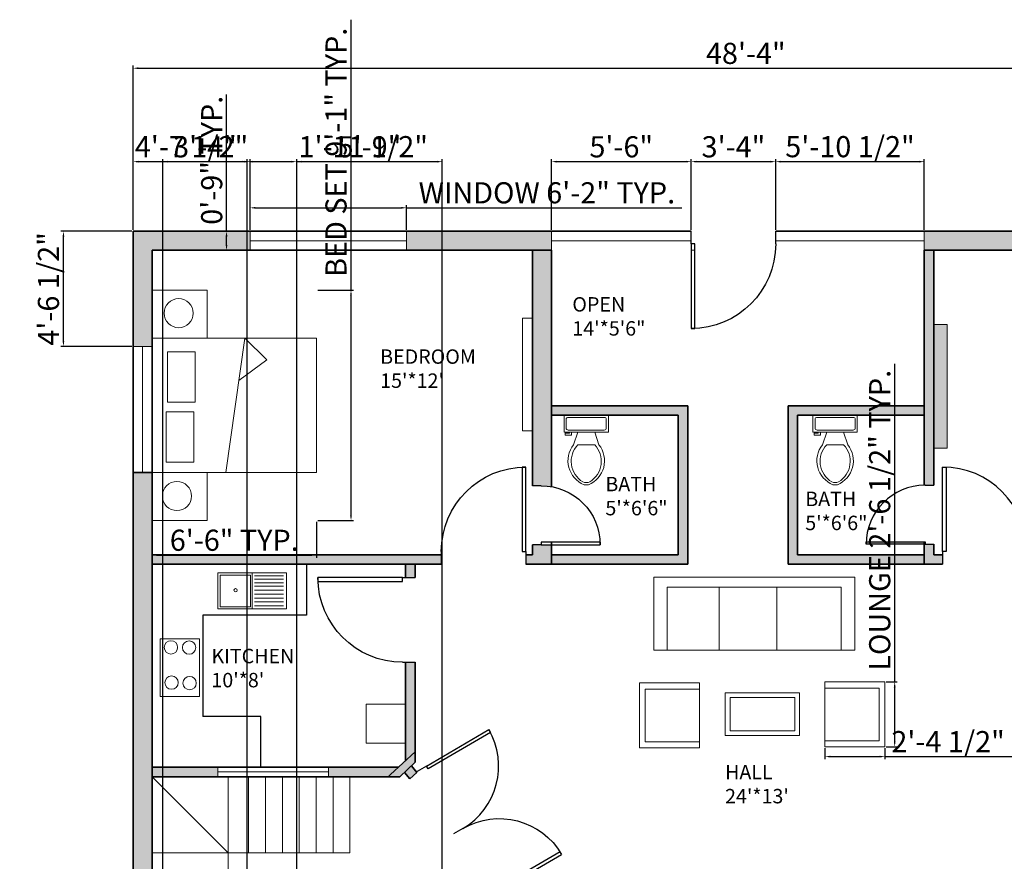
# Model space of a CAD drawing. Units: inches. Extents: x 1433 to 2137, y 2961 to 3626.
# Tile 2 of 3: x 1433 to 1899, y 3228 to 3626. Entities that reach past the tile are written whole.
import ezdxf

# ---------------------------------------------------------------- set-up
doc = ezdxf.new("R2010")
doc.units = ezdxf.units.IN
for name, color, linetype, lineweight in [('A-ANNO-DIMS', 2, 'Continuous', 18), ('A-AREA-IDEN', 7, 'Continuous', 18), ('A-EQPM', 193, 'Continuous', 18), ('A-FLOR-FIXT', 9, 'Continuous', 18), ('A-FLOR-STRS', 7, 'Continuous', 18), ('A-FURN', 8, 'Continuous', 18), ('A-WALL-PATT', 46, 'Continuous', 13), ('bed', 10, 'Continuous', 18), ('door', 50, 'Continuous', 25), ('kit', 193, 'Continuous', 25), ('wall', 46, 'Continuous', 35), ('window', 30, 'Continuous', 18)]:
    doc.layers.add(name, color=color, linetype=linetype, lineweight=lineweight)
doc.styles.get("Standard").update_dxf_attribs({"font": 'arial.ttf'})
doc.dimstyles.new('ISO-25', dxfattribs={"dimtxt": 10, "dimasz": 2.5, "dimexe": 1.25, "dimexo": 0.625, "dimtad": 1, "dimdec": 0, "dimlunit": 4, "dimtxsty": 'Standard', "dimcen": 2.5, "dimadec": 0, "dimazin": 0, "dimtfac": 1, "dimtdec": 0, "dimtmove": 0, "dimatfit": 3, "dimfxl": 1, "dimarcsym": 0})

# ---------------------------------------------------------------- blocks, each defined once
blk = doc.blocks.new('*U2')
for p, q in [((0, 0), (0, -6)), ((40, 0), (40, -6))]:
    blk.add_line(p, q)
blk.add_lwpolyline([(0, 0), (0, 40), (1.75, 40), (1.75, 0)], close=True)
blk.add_arc((0, 0), 40, 0, 90)
blk = doc.blocks.new('*U4')
for p, q in [((9.5, -6), (9.5, -2)), ((-10, -8.5), (-8, -8.5)), ((-10, -9.5), (-10, -8.5)), ((-8, -8.5), (-8, -8)), ((-7, -8), (-7, -9.5)), ((-4, -8), (-6, -14)), ((4, -8), (6, -14)), ((-7, -9.5), (-10, -9.5)), ((4, -14), (-4, -14))]:
    blk.add_line(p, q)
blk.add_lwpolyline([(10.5, -8), (10.5, 0), (-10.5, 0), (-10.5, -8)], close=True)
for points in [[(-9.5, -2), (-9.5, -6)], [(8.5, -1), (-8.5, -1)], [(-8.5, -7), (8.5, -7)]]:
    blk.add_lwpolyline(points)
for centre, radius, start, end in [((-8.62, -1.88), 0.884, 81.8699, 188.1301), ((8.62, -1.88), 0.884, 351.8699, 98.1301), ((-8.62, -6.12), 0.884, 171.8699, 278.1301), ((8.62, -6.12), 0.884, 261.8699, 8.1301), ((3.52, -21.58), 12.17, 141.4691, 247.9714), ((4.2, -21.82), 11.33, 136.3677, 238.9468), ((-3.52, -21.58), 12.17, 292.0284, 38.5307), ((-4.2, -21.82), 11.33, 301.053, 43.6321), ((0, -27.88), 4, 245.7318, 294.2682), ((0, -29), 4, 254.8605, 285.1395)]:
    blk.add_arc(centre, radius, start, end)
blk = doc.blocks.new('*D7')
at = {"layer": 'A-ANNO-DIMS', "color": 0, "lineweight": -2, "transparency": 16777216}
for p, q in [((1486.74, 3526.92), (1486.74, 3604.69)), ((1489.24, 3603.44), (2064.24, 3603.44)), ((2066.74, 3526.92), (2066.74, 3604.69))]:
    blk.add_line(p, q, dxfattribs=at)
at = {"layer": 'A-ANNO-DIMS', "color": 0, "transparency": 16777216}
for points in [[(1489.24, 3603.85), (1489.24, 3603.02), (1486.74, 3603.44)], [(2064.24, 3603.85), (2064.24, 3603.02), (2066.74, 3603.44)]]:
    blk.add_solid(points, dxfattribs=at)
at = {"layer": 'Defpoints', "color": 0, "transparency": 16777216}
for p in [(2066.74, 3603.44), (1486.74, 3526.3), (2066.74, 3526.3)]:
    blk.add_point(p, dxfattribs=at)
at = {"layer": 'A-ANNO-DIMS', "color": 0, "transparency": 16777216, "insert": (1776.74, 3609.17), "char_height": 10, "attachment_point": 5}
blk.add_mtext('48\'-4"', dxfattribs=at)
blk = doc.blocks.new('BED-DOUBLE-SIDE-TABLES')
for p, q in [((34.88, 22.67), (43.9, 86.32)), ((43.9, 86.32), (54.29, 75.94)), ((54.29, 75.94), (41.05, 66.2))]:
    blk.add_line(p, q)
for points in [[(0, 86.32), (26.13, 86.32), (26.13, 108.99), (0, 108.99)], [(0, 22.67), (77.8, 22.67), (77.8, 86.32), (0, 86.32)], [(7.27, 56), (20.39, 56), (20.39, 79.76), (7.27, 79.76)], [(6.72, 27.59), (19.84, 27.59), (19.84, 51.35), (6.72, 51.35)], [(0, 0), (26.13, 0), (26.13, 22.67), (0, 22.67)]]:
    blk.add_lwpolyline(points, close=True)
blk = doc.blocks.new('WIN-EXTERIOR-59_67IN')
blk.add_line((4.5, 0), (4.5, 59.67))
blk.add_lwpolyline([(0, 59.67), (9, 59.67), (9, 0), (0, 0)], close=True)
blk = doc.blocks.new('WIN-EXTERIOR-74_12IN')
blk.add_line((0, 4.5), (74.12, 4.5))
blk.add_lwpolyline([(0, 9), (74.12, 9), (74.12, 0), (0, 0)], close=True)
blk = doc.blocks.new('ARMCHAIR-LOUNGE')
for p, q in [((0, 27.74), (0, 30.73)), ((0, 30.73), (28.38, 30.73)), ((28.38, 30.73), (28.38, 0)), ((0, 0), (0, 2.8)), ((28.38, 0), (0, 0))]:
    blk.add_line(p, q)
blk.add_lwpolyline([(0, 27.74), (0, 2.8), (25.65, 2.8), (25.65, 27.74)], close=True)
blk = doc.blocks.new('*D14')
at = {"layer": 'A-ANNO-DIMS', "color": 0, "lineweight": -2, "transparency": 16777216}
for p, q in [((1589.89, 3498.47), (1589.89, 3626.39)), ((1574.16, 3498.47), (1591.14, 3498.47)), ((1589.89, 3391.99), (1589.89, 3495.97)), ((1574.16, 3389.49), (1591.14, 3389.49))]:
    blk.add_line(p, q, dxfattribs=at)
at = {"layer": 'A-ANNO-DIMS', "color": 0, "transparency": 16777216}
for points in [[(1589.47, 3495.97), (1590.3, 3495.97), (1589.89, 3498.47)], [(1589.47, 3391.99), (1590.3, 3391.99), (1589.89, 3389.49)]]:
    blk.add_solid(points, dxfattribs=at)
at = {"layer": 'Defpoints', "color": 0, "transparency": 16777216}
for p in [(1573.54, 3498.47), (1589.89, 3498.47), (1573.54, 3389.49)]:
    blk.add_point(p, dxfattribs=at)
at = {"layer": 'A-ANNO-DIMS', "color": 0, "transparency": 16777216, "insert": (1584.09, 3563.68), "char_height": 10, "attachment_point": 5, "rotation": 90}
blk.add_mtext('BED SET 9\'-1" TYP.', dxfattribs=at)
blk = doc.blocks.new('*D15')
at = {"layer": 'A-ANNO-DIMS', "color": 0, "lineweight": -2, "transparency": 16777216}
for p, q in [((1495.74, 3388.86), (1495.74, 3371.89)), ((1573.54, 3388.86), (1573.54, 3371.89)), ((1498.24, 3373.14), (1571.04, 3373.14))]:
    blk.add_line(p, q, dxfattribs=at)
at = {"layer": 'A-ANNO-DIMS', "color": 0, "transparency": 16777216}
for points in [[(1498.24, 3373.55), (1498.24, 3372.72), (1495.74, 3373.14)], [(1571.04, 3373.55), (1571.04, 3372.72), (1573.54, 3373.14)]]:
    blk.add_solid(points, dxfattribs=at)
at = {"layer": 'Defpoints', "color": 0, "transparency": 16777216}
for p in [(1495.74, 3389.49), (1573.54, 3389.49), (1573.54, 3373.14)]:
    blk.add_point(p, dxfattribs=at)
at = {"layer": 'A-ANNO-DIMS', "color": 0, "transparency": 16777216, "insert": (1534.64, 3378.87), "char_height": 10, "attachment_point": 5}
blk.add_mtext('6\'-6" TYP.', dxfattribs=at)
blk = doc.blocks.new('*D18')
at = {"layer": 'A-ANNO-DIMS', "color": 0, "lineweight": -2, "transparency": 16777216}
for p, q in [((1542.09, 3526.92), (1542.09, 3538.66)), ((1544.59, 3537.41), (1613.71, 3537.41)), ((1616.21, 3526.92), (1616.21, 3538.66)), ((1616.21, 3537.41), (1746.5, 3537.41))]:
    blk.add_line(p, q, dxfattribs=at)
at = {"layer": 'A-ANNO-DIMS', "color": 0, "transparency": 16777216}
for points in [[(1544.59, 3537.83), (1544.59, 3537), (1542.09, 3537.41)], [(1613.71, 3537.83), (1613.71, 3537), (1616.21, 3537.41)]]:
    blk.add_solid(points, dxfattribs=at)
at = {"layer": 'Defpoints', "color": 0, "transparency": 16777216}
for p in [(1616.21, 3537.41), (1542.09, 3526.3), (1616.21, 3526.3)]:
    blk.add_point(p, dxfattribs=at)
at = {"layer": 'A-ANNO-DIMS', "color": 0, "transparency": 16777216, "insert": (1682.61, 3543.21), "char_height": 10, "attachment_point": 5}
blk.add_mtext('WINDOW 6\'-2" TYP.', dxfattribs=at)
blk = doc.blocks.new('*D19')
at = {"layer": 'A-ANNO-DIMS', "color": 0, "lineweight": -2, "transparency": 16777216}
for p, q in [((1530.98, 3526.3), (1530.98, 3591)), ((1541.47, 3526.3), (1529.73, 3526.3)), ((1530.98, 3519.8), (1530.98, 3523.8)), ((1541.47, 3517.3), (1529.73, 3517.3))]:
    blk.add_line(p, q, dxfattribs=at)
at = {"layer": 'A-ANNO-DIMS', "color": 0, "transparency": 16777216}
for points in [[(1530.56, 3523.8), (1531.39, 3523.8), (1530.98, 3526.3)], [(1530.56, 3519.8), (1531.39, 3519.8), (1530.98, 3517.3)]]:
    blk.add_solid(points, dxfattribs=at)
at = {"layer": 'Defpoints', "color": 0, "transparency": 16777216}
for p in [(1530.98, 3526.3), (1542.09, 3526.3), (1542.09, 3517.3)]:
    blk.add_point(p, dxfattribs=at)
at = {"layer": 'A-ANNO-DIMS', "color": 0, "transparency": 16777216, "insert": (1525.25, 3559.9), "char_height": 10, "attachment_point": 5, "rotation": 90}
blk.add_mtext('0\'-9" TYP.', dxfattribs=at)
blk = doc.blocks.new('*D22')
at = {"layer": 'A-ANNO-DIMS', "color": 0, "lineweight": -2, "transparency": 16777216}
for p, q in [((1847.21, 3313.15), (1847.21, 3463.59)), ((1843.23, 3313.15), (1848.46, 3313.15)), ((1847.21, 3284.92), (1847.21, 3310.65)), ((1843.23, 3282.42), (1848.46, 3282.42))]:
    blk.add_line(p, q, dxfattribs=at)
at = {"layer": 'A-ANNO-DIMS', "color": 0, "transparency": 16777216}
for points in [[(1846.79, 3310.65), (1847.63, 3310.65), (1847.21, 3313.15)], [(1846.79, 3284.92), (1847.63, 3284.92), (1847.21, 3282.42)]]:
    blk.add_solid(points, dxfattribs=at)
at = {"layer": 'Defpoints', "color": 0, "transparency": 16777216}
for p in [(1842.6, 3313.15), (1847.21, 3313.15), (1842.6, 3282.42)]:
    blk.add_point(p, dxfattribs=at)
at = {"layer": 'A-ANNO-DIMS', "color": 0, "transparency": 16777216, "insert": (1841.41, 3389.62), "char_height": 10, "attachment_point": 5, "rotation": 90}
blk.add_mtext('LOUNGE 2\'-6 1/2" TYP.', dxfattribs=at)
blk = doc.blocks.new('*D23')
at = {"layer": 'A-ANNO-DIMS', "color": 0, "lineweight": -2, "transparency": 16777216}
for p, q in [((1814.22, 3281.79), (1814.22, 3276.56)), ((1842.6, 3281.79), (1842.6, 3276.56)), ((1816.72, 3277.81), (1840.1, 3277.81)), ((1842.6, 3277.81), (1930.78, 3277.81))]:
    blk.add_line(p, q, dxfattribs=at)
at = {"layer": 'A-ANNO-DIMS', "color": 0, "transparency": 16777216}
for points in [[(1816.72, 3278.23), (1816.72, 3277.39), (1814.22, 3277.81)], [(1840.1, 3278.23), (1840.1, 3277.39), (1842.6, 3277.81)]]:
    blk.add_solid(points, dxfattribs=at)
at = {"layer": 'Defpoints', "color": 0, "transparency": 16777216}
for p in [(1814.22, 3282.42), (1842.6, 3282.42), (1842.6, 3277.81)]:
    blk.add_point(p, dxfattribs=at)
at = {"layer": 'A-ANNO-DIMS', "color": 0, "transparency": 16777216, "insert": (1887.94, 3283.61), "char_height": 10, "attachment_point": 5}
blk.add_mtext('2\'-4 1/2" TYP.', dxfattribs=at)
blk = doc.blocks.new('*D24')
at = {"layer": 'A-ANNO-DIMS', "color": 0, "lineweight": -2, "transparency": 16777216}
for p, q in [((1486.74, 3526.92), (1486.74, 3560.5)), ((1542.09, 3526.92), (1542.09, 3560.5)), ((1489.24, 3559.25), (1539.59, 3559.25))]:
    blk.add_line(p, q, dxfattribs=at)
at = {"layer": 'A-ANNO-DIMS', "color": 0, "transparency": 16777216}
for points in [[(1489.24, 3559.66), (1489.24, 3558.83), (1486.74, 3559.25)], [(1539.59, 3559.66), (1539.59, 3558.83), (1542.09, 3559.25)]]:
    blk.add_solid(points, dxfattribs=at)
at = {"layer": 'Defpoints', "color": 0, "transparency": 16777216}
for p in [(1542.09, 3559.25), (1486.74, 3526.3), (1542.09, 3526.3)]:
    blk.add_point(p, dxfattribs=at)
at = {"layer": 'A-ANNO-DIMS', "color": 0, "transparency": 16777216, "insert": (1514.42, 3565.04), "char_height": 10, "attachment_point": 5}
blk.add_mtext('4\'-7 1/2"', dxfattribs=at)
blk = doc.blocks.new('*D25')
at = {"layer": 'A-ANNO-DIMS', "color": 0, "lineweight": -2, "transparency": 16777216}
for p, q in [((1684.74, 3526.92), (1684.74, 3560.5)), ((1750.89, 3526.92), (1750.89, 3560.5)), ((1687.24, 3559.25), (1748.39, 3559.25))]:
    blk.add_line(p, q, dxfattribs=at)
at = {"layer": 'A-ANNO-DIMS', "color": 0, "transparency": 16777216}
for points in [[(1687.24, 3559.66), (1687.24, 3558.83), (1684.74, 3559.25)], [(1748.39, 3559.66), (1748.39, 3558.83), (1750.89, 3559.25)]]:
    blk.add_solid(points, dxfattribs=at)
at = {"layer": 'Defpoints', "color": 0, "transparency": 16777216}
for p in [(1750.89, 3559.25), (1684.74, 3526.3), (1750.89, 3526.3)]:
    blk.add_point(p, dxfattribs=at)
at = {"layer": 'A-ANNO-DIMS', "color": 0, "transparency": 16777216, "insert": (1717.81, 3564.98), "char_height": 10, "attachment_point": 5}
blk.add_mtext('5\'-6"', dxfattribs=at)
blk = doc.blocks.new('*D26')
at = {"layer": 'A-ANNO-DIMS', "color": 0, "lineweight": -2, "transparency": 16777216}
for p, q in [((1750.89, 3526.92), (1750.89, 3560.5)), ((1790.89, 3526.92), (1790.89, 3560.5)), ((1753.39, 3559.25), (1788.39, 3559.25))]:
    blk.add_line(p, q, dxfattribs=at)
at = {"layer": 'A-ANNO-DIMS', "color": 0, "transparency": 16777216}
for points in [[(1753.39, 3559.66), (1753.39, 3558.83), (1750.89, 3559.25)], [(1788.39, 3559.66), (1788.39, 3558.83), (1790.89, 3559.25)]]:
    blk.add_solid(points, dxfattribs=at)
at = {"layer": 'Defpoints', "color": 0, "transparency": 16777216}
for p in [(1790.89, 3559.25), (1750.89, 3526.3), (1790.89, 3526.3)]:
    blk.add_point(p, dxfattribs=at)
at = {"layer": 'A-ANNO-DIMS', "color": 0, "transparency": 16777216, "insert": (1770.89, 3564.98), "char_height": 10, "attachment_point": 5}
blk.add_mtext('3\'-4"', dxfattribs=at)
blk = doc.blocks.new('*D27')
at = {"layer": 'A-ANNO-DIMS', "color": 0, "lineweight": -2, "transparency": 16777216}
for p, q in [((1790.89, 3526.92), (1790.89, 3560.5)), ((1861.24, 3526.92), (1861.24, 3560.5)), ((1793.39, 3559.25), (1858.74, 3559.25))]:
    blk.add_line(p, q, dxfattribs=at)
at = {"layer": 'A-ANNO-DIMS', "color": 0, "transparency": 16777216}
for points in [[(1793.39, 3559.66), (1793.39, 3558.83), (1790.89, 3559.25)], [(1858.74, 3559.66), (1858.74, 3558.83), (1861.24, 3559.25)]]:
    blk.add_solid(points, dxfattribs=at)
at = {"layer": 'Defpoints', "color": 0, "transparency": 16777216}
for p in [(1861.24, 3559.25), (1790.89, 3526.3), (1861.24, 3526.3)]:
    blk.add_point(p, dxfattribs=at)
at = {"layer": 'A-ANNO-DIMS', "color": 0, "transparency": 16777216, "insert": (1826.06, 3565.04), "char_height": 10, "attachment_point": 5}
blk.add_mtext('5\'-10 1/2"', dxfattribs=at)
blk = doc.blocks.new('*D32')
at = {"layer": 'A-ANNO-DIMS', "color": 0, "lineweight": -2, "transparency": 16777216}
for p, q in [((1486.11, 3526.3), (1452.54, 3526.3)), ((1453.79, 3474.33), (1453.79, 3523.8)), ((1486.11, 3471.83), (1452.54, 3471.83))]:
    blk.add_line(p, q, dxfattribs=at)
at = {"layer": 'A-ANNO-DIMS', "color": 0, "transparency": 16777216}
for points in [[(1453.37, 3523.8), (1454.21, 3523.8), (1453.79, 3526.3)], [(1453.37, 3474.33), (1454.21, 3474.33), (1453.79, 3471.83)]]:
    blk.add_solid(points, dxfattribs=at)
at = {"layer": 'Defpoints', "color": 0, "transparency": 16777216}
for p in [(1453.79, 3526.3), (1486.74, 3526.3), (1486.74, 3471.83)]:
    blk.add_point(p, dxfattribs=at)
at = {"layer": 'A-ANNO-DIMS', "color": 0, "transparency": 16777216, "insert": (1447.99, 3499.06), "char_height": 10, "attachment_point": 5, "rotation": 90}
blk.add_mtext('4\'-6 1/2"', dxfattribs=at)
blk = doc.blocks.new('*D34')
at = {"layer": 'A-ANNO-DIMS', "color": 0, "lineweight": -2, "transparency": 16777216}
for p, q in [((1500.78, 3055.92), (1500.78, 3560.5)), ((1540.78, 3055.92), (1540.78, 3560.5)), ((1503.28, 3559.25), (1538.28, 3559.25))]:
    blk.add_line(p, q, dxfattribs=at)
at = {"layer": 'A-ANNO-DIMS', "color": 0, "transparency": 16777216}
for points in [[(1503.28, 3559.66), (1503.28, 3558.83), (1500.78, 3559.25)], [(1538.28, 3559.66), (1538.28, 3558.83), (1540.78, 3559.25)]]:
    blk.add_solid(points, dxfattribs=at)
at = {"layer": 'Defpoints', "color": 0, "transparency": 16777216}
for p in [(1540.78, 3559.25), (1500.78, 3055.3), (1540.78, 3055.3)]:
    blk.add_point(p, dxfattribs=at)
at = {"layer": 'A-ANNO-DIMS', "color": 0, "transparency": 16777216, "insert": (1520.78, 3564.98), "char_height": 10, "attachment_point": 5}
blk.add_mtext('3\'-4"', dxfattribs=at)
blk = doc.blocks.new('*D35')
at = {"layer": 'A-ANNO-DIMS', "color": 0, "lineweight": -2, "transparency": 16777216}
for p, q in [((1540.78, 3055.92), (1540.78, 3560.5)), ((1564.19, 3055.92), (1564.19, 3560.5)), ((1543.28, 3559.25), (1561.69, 3559.25)), ((1564.19, 3559.25), (1624.66, 3559.25))]:
    blk.add_line(p, q, dxfattribs=at)
at = {"layer": 'A-ANNO-DIMS', "color": 0, "transparency": 16777216}
for points in [[(1543.28, 3559.66), (1543.28, 3558.83), (1540.78, 3559.25)], [(1561.69, 3559.66), (1561.69, 3558.83), (1564.19, 3559.25)]]:
    blk.add_solid(points, dxfattribs=at)
at = {"layer": 'Defpoints', "color": 0, "transparency": 16777216}
for p in [(1564.19, 3559.25), (1540.78, 3055.3), (1564.19, 3055.3)]:
    blk.add_point(p, dxfattribs=at)
at = {"layer": 'A-ANNO-DIMS', "color": 0, "transparency": 16777216, "insert": (1595.68, 3565.04), "char_height": 10, "attachment_point": 5}
blk.add_mtext('1\'-11 1/2"', dxfattribs=at)
blk = doc.blocks.new('*D36')
at = {"layer": 'A-ANNO-DIMS', "color": 0, "lineweight": -2, "transparency": 16777216}
for p, q in [((1564.19, 3055.92), (1564.19, 3560.5)), ((1633.11, 3055.92), (1633.11, 3560.5)), ((1566.69, 3559.25), (1630.61, 3559.25))]:
    blk.add_line(p, q, dxfattribs=at)
at = {"layer": 'A-ANNO-DIMS', "color": 0, "transparency": 16777216}
for points in [[(1566.69, 3559.66), (1566.69, 3558.83), (1564.19, 3559.25)], [(1630.61, 3559.66), (1630.61, 3558.83), (1633.11, 3559.25)]]:
    blk.add_solid(points, dxfattribs=at)
at = {"layer": 'Defpoints', "color": 0, "transparency": 16777216}
for p in [(1633.11, 3559.25), (1564.19, 3055.3), (1633.11, 3055.3)]:
    blk.add_point(p, dxfattribs=at)
at = {"layer": 'A-ANNO-DIMS', "color": 0, "transparency": 16777216, "insert": (1598.65, 3564.98), "char_height": 10, "attachment_point": 5}
blk.add_mtext('5\'-9"', dxfattribs=at)

msp = doc.modelspace()

# ---------------------------------------------------------------- hatches: boundary and pattern name
at = {"layer": 'A-WALL-PATT'}
h = msp.add_hatch(color=256, dxfattribs=at)
h.dxf.hatch_style = 1
h.paths.add_polyline_path([(1542.09, 3517.3), (1542.09, 3526.3), (1486.74, 3526.3), (1486.74, 3471.83), (1495.74, 3471.83), (1495.74, 3475.8), (1495.74, 3498.47), (1495.74, 3517.3)])
h = msp.add_hatch(color=256, dxfattribs=at)
h.dxf.hatch_style = 1
h.paths.add_polyline_path([(1542.09, 3526.3), (1486.74, 3526.3), (1486.74, 3471.83), (1495.74, 3471.83), (1495.74, 3475.8), (1495.74, 3517.3), (1542.09, 3517.3)])
h.paths.add_polyline_path([(2066.74, 3526.3), (2012.26, 3526.3), (2012.26, 3517.3), (2057.74, 3517.3), (2057.74, 3472.19), (2066.74, 3472.19)])
h.paths.add_polyline_path([(2066.74, 3412.52), (2057.74, 3412.52), (2057.74, 3389.96), (2057.74, 3324.56), (2066.74, 3324.56)])
h.paths.add_polyline_path([(2066.74, 3264.89), (2057.74, 3264.89), (2057.74, 3238.24), (2057.74, 3215.57), (2057.74, 3212.8), (2057.74, 3154.53), (2066.74, 3154.53)])
h = msp.add_hatch(color=256, dxfattribs=at)
h.dxf.hatch_style = 1
h.paths.add_polyline_path([(1684.74, 3526.3), (1616.21, 3526.3), (1616.21, 3517.3), (1684.74, 3517.3)])
h.paths.add_polyline_path([(1938.14, 3526.3), (1861.24, 3526.3), (1861.24, 3517.3), (1938.14, 3517.3)])
h = msp.add_hatch(color=256, dxfattribs=at)
h.dxf.hatch_style = 1
h.paths.add_polyline_path([(1684.74, 3517.3), (1675.74, 3517.3), (1675.74, 3405.93), (1679.92, 3405.93, -0.043454), (1684.74, 3405.51)])
h.paths.add_polyline_path([(1861.24, 3373.3), (1801.24, 3373.3), (1801.24, 3439.3), (1861.24, 3439.3), (1861.24, 3443.8), (1796.74, 3443.8), (1796.74, 3368.8), (1861.24, 3368.8)])
h.paths.add_polyline_path([(1749.24, 3443.8), (1684.74, 3443.8), (1684.74, 3439.3), (1744.74, 3439.3), (1744.74, 3373.3), (1684.74, 3373.3), (1684.74, 3368.8), (1749.24, 3368.8)])
h.paths.add_polyline_path([(1684.74, 3378.05), (1679.92, 3378.05), (1675.74, 3378.05), (1675.74, 3373.3), (1672.64, 3373.3), (1672.64, 3368.8), (1684.74, 3368.8), (1684.74, 3373.3)])
h.paths.add_polyline_path([(1865.74, 3378.26), (1861.56, 3378.26), (1861.24, 3378.26), (1861.24, 3368.8), (1869.81, 3368.8), (1869.81, 3373.3), (1865.74, 3373.3)])
h.paths.add_polyline_path([(2057.74, 3373.3), (1909.81, 3373.3), (1909.81, 3368.8), (2057.74, 3368.8)])
h.paths.add_polyline_path([(1919.74, 3368.8), (1915.24, 3368.8), (1915.24, 3366.92), (1919.74, 3366.92)])
h.paths.add_polyline_path([(1919.74, 3326.92), (1915.24, 3326.92), (1915.24, 3308.14), (1919.74, 3308.14)])
h.paths.add_polyline_path([(1919.74, 3236.84), (1915.24, 3236.84), (1915.24, 3212.8), (1919.74, 3212.8)])
h.paths.add_polyline_path([(1859.74, 3208.3), (1855.24, 3208.3), (1855.24, 3203.85), (1855.29, 3203.85), (1859.74, 3203.85)])
h = msp.add_hatch(color=256, dxfattribs=at)
h.dxf.hatch_style = 1
h.paths.add_polyline_path([(1833.71, 3379.48), (1861.56, 3379.48), (1861.56, 3378.26), (1833.68, 3378.26), (1833.68, 3379.48), (1833.71, 3379.48, -0.398142), (1861.24, 3406.14), (1861.24, 3517.3), (1865.74, 3517.3), (1865.74, 3482.28), (1871.97, 3482.28), (1871.97, 3423.64), (1865.74, 3423.64), (1865.74, 3406.14), (1861.56, 3406.14, 0.401453)])
h = msp.add_hatch(color=256, dxfattribs=at)
h.dxf.hatch_style = 1
h.paths.add_polyline_path([(1500.78, 3055.3), (1486.74, 3055.3), (1486.74, 3046.3), (1500.78, 3046.3), (1500.78, 3049.3)])
h.paths.add_polyline_path([(1495.74, 3412.16), (1486.74, 3412.16), (1486.74, 3055.3), (1495.74, 3055.3)])
h = msp.add_hatch(color=256, dxfattribs=at)
h.dxf.hatch_style = 1
h.paths.add_polyline_path([(1632.64, 3373.3), (1495.74, 3373.3), (1495.74, 3368.8), (1632.64, 3368.8)])
h.paths.add_polyline_path([(1620.24, 3368.8), (1615.74, 3368.8), (1615.74, 3362.47), (1620.24, 3362.47)])
h.paths.add_polyline_path([(1526.85, 3272.8), (1495.74, 3272.8), (1495.74, 3268.3), (1526.85, 3268.3)])
h.paths.add_polyline_path([(1612.35, 3272.8), (1579.17, 3272.8), (1579.17, 3268.3), (1607.43, 3268.3), (1608.56, 3269.33)])
h.paths.add_polyline_path([(1620.24, 3275.2), (1620.24, 3280), (1608.56, 3269.33), (1607.43, 3268.3), (1613.07, 3268.3)])
h.paths.add_polyline_path([(1620.24, 3322.47), (1615.74, 3322.47), (1615.74, 3275.89), (1620.24, 3280)])
h.paths.add_polyline_path([(1621.12, 3270.32), (1618.48, 3273.5), (1615.2, 3270.34), (1617.74, 3267.34)])
h.paths.add_polyline_path([(1658.27, 3208.55), (1655.63, 3211.74), (1652.35, 3208.58), (1654.95, 3205.51)])
h.paths.add_polyline_path([(1564.19, 3050.13), (1564.19, 3055.3), (1540.78, 3055.3), (1540.78, 3049.3, -0.01877), (1540.67, 3046.3), (1564.19, 3046.3)])
h.paths.add_polyline_path([(1693.15, 3055.3), (1655.74, 3055.3), (1633.11, 3055.3), (1633.11, 3050.13), (1633.11, 3046.3), (1693.15, 3046.3)])
h.paths.add_polyline_path([(1804.24, 3127.3), (1804.24, 3208.3), (1799.74, 3208.3), (1799.74, 3131.8), (1799.74, 3055.3), (1804.24, 3055.3)])
h.paths.add_polyline_path([(1655.74, 3142.86), (1651.24, 3142.86), (1651.24, 3055.3), (1655.74, 3055.3)])
h.paths.add_polyline_path([(2057.74, 3212.8), (1903.59, 3212.8), (1903.59, 3208.3), (2057.74, 3208.3)])
h.paths.add_polyline_path([(1855.24, 3055.3), (1855.24, 3046.3), (2066.74, 3046.3), (2066.74, 3094.86), (2057.74, 3094.86), (2057.74, 3094.45), (2057.74, 3071.77), (2057.74, 3055.3)])

# ---------------------------------------------------------------- linework, layer by layer
at = {"layer": 'A-EQPM'}
for points in [[(1499.54, 3333.52), (1518.18, 3333.52), (1518.18, 3306.3), (1499.54, 3306.3)], [(1615.74, 3302.61), (1597.02, 3302.61), (1597.02, 3284.13), (1615.74, 3284.13)]]:
    msp.add_lwpolyline(points, close=True, dxfattribs=at)
for centre in [(1504.68, 3329.49), (1513.26, 3329.41), (1504.97, 3312.8), (1513.52, 3312.59)]:
    msp.add_circle(centre, 3.15, dxfattribs=at)
at = {"layer": 'A-FLOR-FIXT'}
for p, q in [((1543.11, 3364.79), (1543.11, 3347.67)), ((1544.24, 3363.36), (1557.95, 3363.36)), ((1544.24, 3361.71), (1557.95, 3361.71)), ((1544.24, 3359.99), (1557.95, 3359.99)), ((1544.24, 3358.38), (1557.95, 3358.38)), ((1544.24, 3356.5), (1557.95, 3356.5)), ((1544.24, 3354.73), (1557.95, 3354.73)), ((1544.24, 3352.81), (1557.95, 3352.81)), ((1544.24, 3350.97), (1557.95, 3350.97)), ((1544.24, 3349.13), (1557.95, 3349.13))]:
    msp.add_line(p, q, dxfattribs=at)
for points in [[(1526.86, 3364.79), (1559.37, 3364.79), (1559.37, 3347.67), (1526.86, 3347.67)], [(1527.96, 3363.67), (1542.39, 3363.67), (1542.39, 3348.71), (1527.96, 3348.71)]]:
    msp.add_lwpolyline(points, close=True, dxfattribs=at)
msp.add_circle((1535.24, 3356.52), 0.768, dxfattribs=at)
at = {"layer": 'A-FLOR-STRS'}
for p, q in [((1531.74, 3232.3), (1495.74, 3268.3)), ((1531.74, 3232.3), (1531.74, 3268.3)), ((1541.39, 3268.3), (1541.39, 3232.3)), ((1549.39, 3268.3), (1549.39, 3232.3)), ((1557.39, 3268.3), (1557.39, 3232.3)), ((1565.39, 3268.3), (1565.39, 3232.3)), ((1573.39, 3268.3), (1573.39, 3232.3)), ((1581.39, 3268.3), (1581.39, 3232.3)), ((1589.39, 3268.3), (1589.39, 3232.3)), ((1589.39, 3244.3), (1589.39, 3232.3)), ((1531.74, 3232.3), (1495.74, 3232.3)), ((1589.39, 3232.3), (1531.74, 3232.3)), ((1531.74, 3144.3), (1531.74, 3232.3))]:
    msp.add_line(p, q, dxfattribs=at)
at = {"layer": 'A-FURN'}
for p, q in [((1733.15, 3328.13), (1733.15, 3362.73)), ((1733.15, 3362.73), (1733.15, 3362.73)), ((1733.15, 3362.73), (1828.27, 3362.73)), ((1828.27, 3362.73), (1828.27, 3328.13)), ((1764.08, 3357.98), (1764.08, 3328.13)), ((1791.49, 3357.98), (1791.49, 3328.13)), ((1739.46, 3328.13), (1733.15, 3328.13)), ((1828.27, 3328.13), (1815.92, 3328.13))]:
    msp.add_line(p, q, dxfattribs=at)
for points in [[(1675.74, 3485.15), (1671.04, 3485.15), (1671.04, 3431.91), (1675.74, 3431.91)], [(1865.74, 3423.64), (1871.97, 3423.64), (1871.97, 3482.28), (1865.74, 3482.28)], [(1739.46, 3357.98), (1739.46, 3328.13), (1821.86, 3328.13), (1821.86, 3357.98)], [(1767.03, 3287.78), (1767.03, 3308.05), (1802.18, 3308.05), (1802.18, 3287.78)], [(1769.3, 3290.05), (1769.3, 3305.78), (1799.91, 3305.78), (1799.91, 3290.05)]]:
    msp.add_lwpolyline(points, close=True, dxfattribs=at)
at = {"layer": 'bed'}
for centre in [(1508.33, 3487.58), (1507.51, 3401.08)]:
    msp.add_circle(centre, 6.9, dxfattribs=at)
at = {"layer": 'kit'}
for p, q in [((1495.74, 3368.8), (1519.74, 3368.8)), ((1568.77, 3368.8), (1568.77, 3344.8)), ((1568.77, 3344.8), (1519.74, 3344.8)), ((1519.74, 3344.8), (1519.74, 3296.8)), ((1547.19, 3296.8), (1519.74, 3296.8)), ((1547.19, 3272.8), (1547.19, 3296.8))]:
    msp.add_line(p, q, dxfattribs=at)
at = {"layer": 'wall'}
for p, q in [((1486.74, 3526.3), (1750.89, 3526.3)), ((1486.74, 3046.3), (1486.74, 3526.3)), ((1790.89, 3526.3), (2066.74, 3526.3)), ((1495.74, 3517.3), (1684.74, 3517.3)), ((1495.74, 3055.3), (1495.74, 3517.3)), ((1495.74, 3517.3), (1495.74, 3373.3)), ((1675.74, 3405.93), (1675.74, 3517.3)), ((1684.74, 3405.51), (1684.74, 3517.3)), ((1861.24, 3517.3), (1861.24, 3406.14)), ((1861.24, 3517.3), (2057.74, 3517.3)), ((2057.74, 3517.3), (1865.74, 3517.3)), ((1865.74, 3517.3), (1865.74, 3406.14)), ((1749.24, 3443.8), (1684.74, 3443.8)), ((1744.74, 3439.3), (1684.74, 3439.3)), ((1744.74, 3373.3), (1744.74, 3439.3)), ((1749.24, 3368.8), (1749.24, 3443.8)), ((1796.74, 3368.8), (1796.74, 3443.8)), ((1796.74, 3443.8), (1861.24, 3443.8)), ((1801.24, 3373.3), (1801.24, 3439.3)), ((1801.24, 3439.3), (1861.24, 3439.3)), ((1684.74, 3368.8), (1684.74, 3379.27)), ((1861.24, 3379.48), (1861.24, 3368.8)), ((1675.74, 3373.3), (1675.74, 3378.05)), ((1865.74, 3378.26), (1865.74, 3373.3)), ((1495.74, 3373.3), (1632.64, 3373.3)), ((1672.64, 3373.3), (1675.74, 3373.3)), ((1684.74, 3373.3), (1744.74, 3373.3)), ((1861.24, 3373.3), (1801.24, 3373.3)), ((1865.74, 3373.3), (1869.81, 3373.3)), ((1495.74, 3368.8), (1632.64, 3368.8)), ((1495.74, 3368.8), (1495.74, 3272.8)), ((1615.74, 3362.47), (1615.74, 3368.8)), ((1620.24, 3362.47), (1620.24, 3368.8)), ((1672.64, 3368.8), (1684.74, 3368.8)), ((1684.74, 3368.8), (1749.24, 3368.8)), ((1861.24, 3368.8), (1796.74, 3368.8)), ((1861.24, 3368.8), (1869.81, 3368.8)), ((1615.74, 3275.89), (1615.74, 3322.47)), ((1620.24, 3275.2), (1620.24, 3322.47)), ((1608.56, 3269.33), (1620.24, 3280)), ((1495.74, 3272.8), (1612.35, 3272.8)), ((1613.06, 3268.28), (1620.24, 3275.2)), ((1621.12, 3270.32), (1618.48, 3273.5)), ((1495.74, 3268.3), (1613.07, 3268.3)), ((1608.56, 3269.33), (1607.43, 3268.3)), ((1615.2, 3270.34), (1617.74, 3267.34)), ((1617.74, 3267.34), (1621.12, 3270.32)), ((1621.17, 3270.77), (1620.88, 3270.61))]:
    msp.add_line(p, q, dxfattribs=at)
msp.add_lwpolyline([(1486.74, 3412.16), (1495.74, 3412.16), (1495.74, 3055.3), (1486.74, 3055.3)], close=True, dxfattribs=at)
at = {"layer": 'window'}
for p, q in [((1684.74, 3517.3), (1684.74, 3526.3)), ((1861.24, 3517.3), (1861.24, 3526.3)), ((1684.74, 3521.8), (1750.89, 3521.8)), ((1790.78, 3521.8), (1861.24, 3521.8)), ((1750.89, 3517.3), (1752.64, 3517.3)), ((1526.85, 3270.55), (1579.17, 3270.55))]:
    msp.add_line(p, q, dxfattribs=at)
msp.add_lwpolyline([(1526.85, 3272.8), (1579.17, 3272.8), (1579.17, 3268.3), (1526.85, 3268.3)], close=True, dxfattribs=at)

# ---------------------------------------------------------------- block references
at = {"layer": 'A-FLOR-FIXT'}
for p in [(1701.23, 3439.3), (1819.03, 3439.3)]:
    msp.add_blockref('*U4', p, dxfattribs=at)
at = {"layer": 'A-FURN', "extrusion": (0, 0, -1), "zscale": -1}
msp.add_blockref('ARMCHAIR-LOUNGE', (-1754.84, 3282.04), dxfattribs=at)
at = {"layer": 'A-FURN'}
msp.add_blockref('ARMCHAIR-LOUNGE', (1814.22, 3282.42), dxfattribs=at)
at = {"layer": 'bed'}
msp.add_blockref('BED-DOUBLE-SIDE-TABLES', (1495.74, 3389.49), dxfattribs=at)
at = {"layer": 'door', "xscale": -1}
for p, rotation in [((1750.89, 3520.3), 180), ((1614.24, 3362.47), 90)]:
    msp.add_blockref('*U2', p, dxfattribs=dict(at, rotation=rotation))
msp.add_blockref('*U2', (1672.64, 3374.8), dxfattribs=at)
at = {"layer": 'door'}
msp.add_blockref('*U2', (1869.81, 3374.8), dxfattribs=at)
for p, xscale, yscale, zscale, rotation in [((1679.92, 3378.05), -0.6969495689774577, 0.6969495689774577, 0.6969495689774577, 270), ((1861.56, 3378.26), 0.6969495689774577, 0.6969495689774577, 0.6969495689774577, 90.00000000000003), ((1625.59, 3273.35), 0.8544553422168171, 0.8544553422168171, 0.8544553422168171, 300.2802112171161), ((1660.06, 3214.32), -0.8544553422168171, 0.8544553422168171, 0.8544553422168168, 300.2802112171161)]:
    msp.add_blockref('*U2', p, dxfattribs=dict(at, xscale=xscale, yscale=yscale, zscale=zscale, rotation=rotation))
at = {"layer": 'window'}
for name, p in [('WIN-EXTERIOR-74_12IN', (1542.09, 3517.3)), ('WIN-EXTERIOR-59_67IN', (1486.74, 3412.16))]:
    msp.add_blockref(name, p, dxfattribs=at)

# ---------------------------------------------------------------- texts
at = {"layer": 'A-AREA-IDEN', "char_height": 6.823, "attachment_point": 1}
for s, insert in [('OPEN\\P14\'*5\'6"', (1694.64, 3495.16)), ("BEDROOM\\P15'*12'", (1603.69, 3470.44)), ('BATH\\P5\'*6\'6"', (1710.29, 3410.15)), ('BATH\\P5\'*6\'6"', (1804.89, 3403.14)), ("KITCHEN\\P10'*8'", (1523.82, 3328.79)), ("HALL\\P24'*13'", (1766.93, 3273.9))]:
    msp.add_mtext_dynamic_manual_height_columns(s, width=135.668, gutter_width=34.12, heights=[0], dxfattribs=dict(at, insert=insert))

# ---------------------------------------------------------------- dimensions: what is measured, and where the dimension line sits
at = {"layer": 'A-ANNO-DIMS'}
for base, p1, p2, text, picture, middle in [((1589.89, 3498.47), (1573.54, 3389.49), (1573.54, 3498.47), 'BED SET <> TYP.', '*D14', (1584.09, 3563.68)), ((1530.98, 3526.3), (1542.09, 3517.3), (1542.09, 3526.3), '<> TYP.', '*D19', (1525.25, 3559.9)), ((1847.21, 3313.15), (1842.6, 3282.42), (1842.6, 3313.15), 'LOUNGE <> TYP.', '*D22', (1841.41, 3389.62))]:
    dim = msp.add_linear_dim(base=base, p1=p1, p2=p2, angle=90, text=text, dimstyle='ISO-25', override={"dimdec": 1, "dimlfac": 1, "dimrnd": 0, "dimzin": 1, "dimdsep": 46, "dimlunit": 4, "dimfrac": 2}, dxfattribs=at)
    dim.commit()
    dim.dimension.update_dxf_attribs({"geometry": picture, "text_midpoint": middle})
for base, p1, p2, override, picture, middle in [((2066.74, 3603.44), (1486.74, 3526.3), (2066.74, 3526.3), {"dimclrd": 0, "dimclre": 0, "dimclrt": 0}, '*D7', (1776.74, 3609.17)), ((1542.0943, 3559.2469), (1486.7395, 3526.2969), (1542.0943, 3526.2969), {"dimdec": 1, "dimlfac": 1, "dimrnd": 0, "dimzin": 1, "dimdsep": 46, "dimlunit": 4, "dimfrac": 2}, '*D24', (1514.4169, 3565.0425)), ((1564.19, 3559.25), (1540.78, 3055.3), (1564.19, 3055.3), {"dimdec": 1, "dimlfac": 1, "dimrnd": 0, "dimzin": 1, "dimdsep": 46, "dimlunit": 4, "dimfrac": 2}, '*D35', (1595.68, 3565.04)), ((1861.2395, 3559.2469), (1790.8902, 3526.2969), (1861.2395, 3526.2969), {"dimdec": 1, "dimlfac": 1, "dimrnd": 0, "dimzin": 1, "dimdsep": 46, "dimlunit": 4, "dimfrac": 2}, '*D27', (1826.0648, 3565.0425)), ((1540.78, 3559.25), (1500.78, 3055.3), (1540.78, 3055.3), {"dimdec": 1, "dimlfac": 1, "dimrnd": 0, "dimzin": 1, "dimdsep": 46, "dimlunit": 4, "dimfrac": 2}, '*D34', (1520.78, 3564.98)), ((1633.11, 3559.25), (1564.19, 3055.3), (1633.11, 3055.3), {"dimdec": 1, "dimlfac": 1, "dimrnd": 0, "dimzin": 1, "dimdsep": 46, "dimlunit": 4, "dimfrac": 2}, '*D36', (1598.65, 3564.98)), ((1750.8902, 3559.2469), (1684.7395, 3526.2969), (1750.8902, 3526.2969), {"dimdec": 1, "dimlfac": 1, "dimrnd": 0, "dimzin": 1, "dimdsep": 46, "dimlunit": 4, "dimfrac": 2}, '*D25', (1717.8148, 3564.9777)), ((1790.89, 3559.25), (1750.89, 3526.3), (1790.89, 3526.3), {"dimdec": 1, "dimlfac": 1, "dimrnd": 0, "dimzin": 1, "dimdsep": 46, "dimlunit": 4, "dimfrac": 2}, '*D26', (1770.89, 3564.98))]:
    dim = msp.add_linear_dim(base=base, p1=p1, p2=p2, dimstyle='ISO-25', override=override, dxfattribs=at)
    dim.commit()
    dim.dimension.update_dxf_attribs({"geometry": picture, "text_midpoint": middle})
for base, p1, p2, text, picture, middle in [((1616.21, 3537.41), (1542.09, 3526.3), (1616.21, 3526.3), 'WINDOW <> TYP.', '*D18', (1682.61, 3543.21)), ((1573.54, 3373.14), (1495.74, 3389.49), (1573.54, 3389.49), '<> TYP.', '*D15', (1534.64, 3378.87)), ((1842.6, 3277.81), (1814.22, 3282.42), (1842.6, 3282.42), '<> TYP.', '*D23', (1887.94, 3283.61))]:
    dim = msp.add_linear_dim(base=base, p1=p1, p2=p2, text=text, dimstyle='ISO-25', override={"dimdec": 1, "dimlfac": 1, "dimrnd": 0, "dimzin": 1, "dimdsep": 46, "dimlunit": 4, "dimfrac": 2}, dxfattribs=at)
    dim.commit()
    dim.dimension.update_dxf_attribs({"geometry": picture, "text_midpoint": middle})
dim = msp.add_linear_dim(base=(1453.79, 3526.3), p1=(1486.74, 3471.83), p2=(1486.74, 3526.3), angle=90, dimstyle='ISO-25', override={"dimdec": 1, "dimlfac": 1, "dimrnd": 0, "dimzin": 1, "dimdsep": 46, "dimlunit": 4, "dimfrac": 2}, dxfattribs=at)
dim.commit()
dim.dimension.update_dxf_attribs({"geometry": '*D32', "text_midpoint": (1447.99, 3499.06)})

doc.saveas('drawing.dxf')
